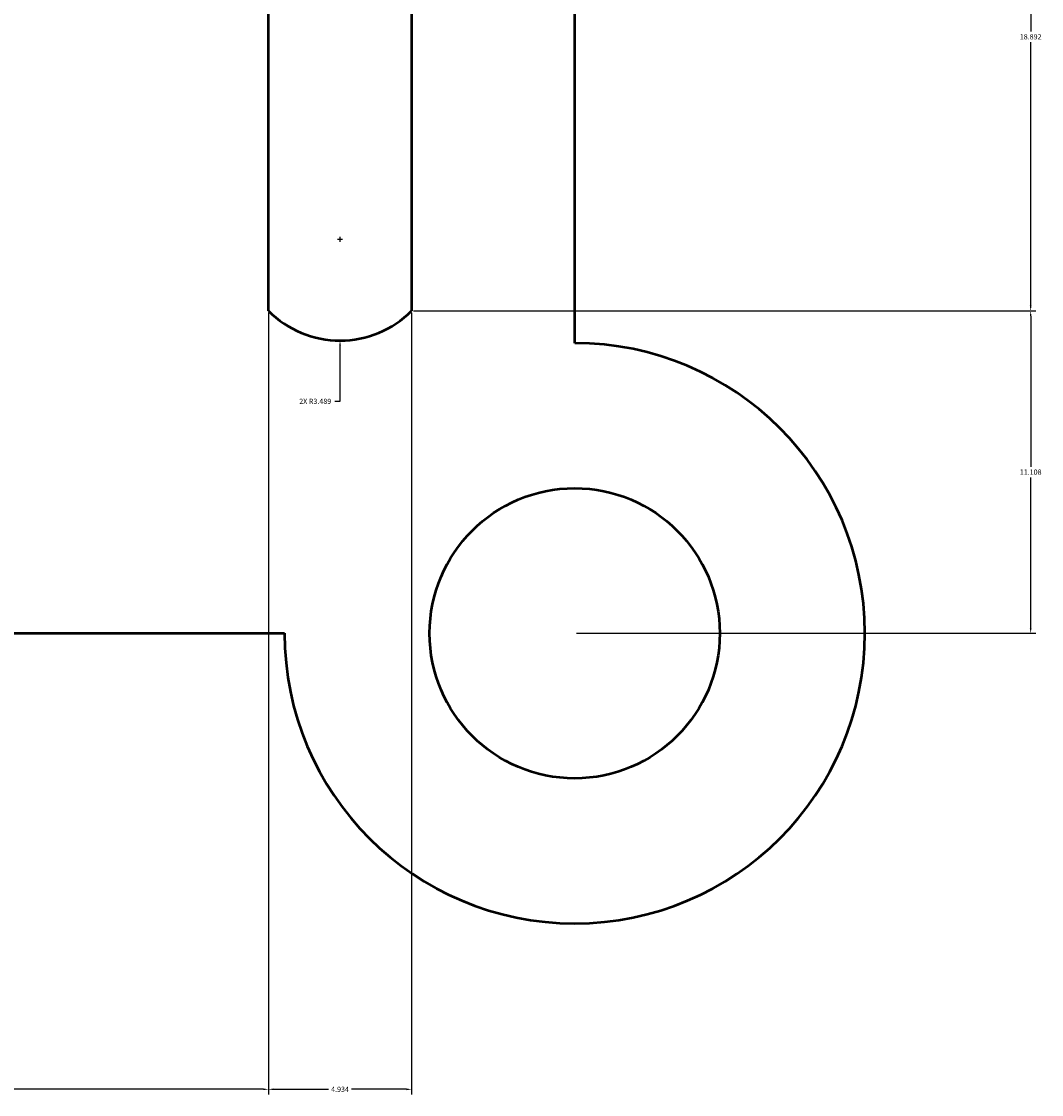
# Model space of a CAD drawing. Units: inches. Extents: x -14 to 108, y -9 to 83.
# Tile 8 of 13: x 73 to 108, y -9 to 28. Entities that reach past the tile are written whole.
import ezdxf

# ---------------------------------------------------------------- set-up
doc = ezdxf.new("R2010")
doc.units = ezdxf.units.IN
doc.header["$MEASUREMENT"] = 0
doc.layers.add('M-DIMS', color=2, linetype='Continuous', lineweight=18)
doc.layers.add('M-OUTL', color=7, linetype='Continuous', lineweight=50)
doc.styles.get("Standard").update_dxf_attribs({"font": 'arial.ttf'})
doc.dimstyles.get("Standard").update_dxf_attribs({"dimtxt": 0.18, "dimasz": 0.18, "dimexe": 0.18, "dimexo": 0.0625, "dimgap": 0.09, "dimtad": 0, "dimtih": 1, "dimtoh": 1, "dimzin": 0, "dimdsep": 46, "dimtxsty": 'Standard', "dimcen": 0.09, "dimadec": 0, "dimazin": 0, "dimtfac": 1, "dimtofl": 0, "dimtmove": 0, "dimatfit": 3, "dimfxl": 1, "dimtolj": 1, "dimtzin": 0, "dimarcsym": 0})

# ---------------------------------------------------------------- blocks, each defined once
blk = doc.blocks.new('SLOT-VERTICAL')
for points in [[(0, 1.021), (0, 40.458)], [(4.933, 40.458), (4.933, 1.021)]]:
    blk.add_lwpolyline(points)
blk.add_arc((2.466, 3.488), 3.489, 225, 315)
blk = doc.blocks.new('HOLE-D10')
blk.add_circle((5, 5), 5)
blk = doc.blocks.new('*D8')
at = {"layer": 'Defpoints', "color": 0, "transparency": 16777216}
for p in [(47.098, 37.119), (81.545, 18.227), (81.545, -8.596)]:
    blk.add_point(p, dxfattribs=at)
at = {"layer": 'M-DIMS', "color": 0, "lineweight": -2, "transparency": 16777216}
for p, q in [((47.098, 37.057), (47.098, -8.776)), ((81.545, 18.165), (81.545, -8.776)), ((47.278, -8.596), (63.927, -8.596)), ((81.365, -8.596), (64.716, -8.596))]:
    blk.add_line(p, q, dxfattribs=at)
at = {"layer": 'M-DIMS', "color": 0, "transparency": 16777216}
for points in [[(47.278, -8.566), (47.278, -8.626), (47.098, -8.596)], [(81.365, -8.566), (81.365, -8.626), (81.545, -8.596)]]:
    blk.add_solid(points, dxfattribs=at)
at = {"layer": 'M-DIMS', "color": 0, "transparency": 16777216, "insert": (64.321, -8.596), "char_height": 0.18, "attachment_point": 5}
blk.add_mtext('\\A1;34.45', dxfattribs=at)
blk = doc.blocks.new('*D9')
at = {"layer": 'Defpoints', "color": 0, "transparency": 16777216}
for p in [(81.545, 18.227), (86.478, 18.227), (86.478, -8.596)]:
    blk.add_point(p, dxfattribs=at)
at = {"layer": 'M-DIMS', "color": 0, "lineweight": -2, "transparency": 16777216}
for p, q in [((81.545, 18.165), (81.545, -8.776)), ((86.478, 18.165), (86.478, -8.776)), ((81.725, -8.596), (83.615, -8.596)), ((86.298, -8.596), (84.408, -8.596))]:
    blk.add_line(p, q, dxfattribs=at)
at = {"layer": 'M-DIMS', "color": 0, "transparency": 16777216}
for points in [[(81.725, -8.566), (81.725, -8.626), (81.545, -8.596)], [(86.298, -8.566), (86.298, -8.626), (86.478, -8.596)]]:
    blk.add_solid(points, dxfattribs=at)
at = {"layer": 'M-DIMS', "color": 0, "transparency": 16777216, "insert": (84.011, -8.596), "char_height": 0.18, "attachment_point": 5}
blk.add_mtext('\\A1;4.934', dxfattribs=at)
blk = doc.blocks.new('*D10')
at = {"layer": 'Defpoints', "color": 0, "transparency": 16777216}
for p in [(86.478, 18.227), (107.813, 18.227), (92.098, 7.119)]:
    blk.add_point(p, dxfattribs=at)
at = {"layer": 'M-DIMS', "color": 0, "lineweight": -2, "transparency": 16777216}
for p, q in [((86.541, 18.227), (107.993, 18.227)), ((107.813, 18.047), (107.813, 12.855)), ((107.813, 7.299), (107.813, 12.491)), ((92.16, 7.119), (107.993, 7.119))]:
    blk.add_line(p, q, dxfattribs=at)
at = {"layer": 'M-DIMS', "color": 0, "transparency": 16777216}
for points in [[(107.783, 18.047), (107.843, 18.047), (107.813, 18.227)], [(107.783, 7.299), (107.843, 7.299), (107.813, 7.119)]]:
    blk.add_solid(points, dxfattribs=at)
at = {"layer": 'M-DIMS', "color": 0, "transparency": 16777216, "insert": (107.813, 12.673), "char_height": 0.18, "attachment_point": 5}
blk.add_mtext('\\A1;11.108', dxfattribs=at)
blk = doc.blocks.new('*D11')
at = {"layer": 'Defpoints', "color": 0, "transparency": 16777216}
for p in [(47.098, 37.119), (107.813, 37.119), (86.478, 18.227)]:
    blk.add_point(p, dxfattribs=at)
at = {"layer": 'M-DIMS', "color": 0, "lineweight": -2, "transparency": 16777216}
for p, q in [((47.16, 37.119), (107.993, 37.119)), ((107.813, 36.939), (107.813, 27.855)), ((107.813, 18.407), (107.813, 27.491)), ((86.541, 18.227), (107.993, 18.227))]:
    blk.add_line(p, q, dxfattribs=at)
at = {"layer": 'M-DIMS', "color": 0, "transparency": 16777216}
for points in [[(107.783, 36.939), (107.843, 36.939), (107.813, 37.119)], [(107.783, 18.407), (107.843, 18.407), (107.813, 18.227)]]:
    blk.add_solid(points, dxfattribs=at)
at = {"layer": 'M-DIMS', "color": 0, "transparency": 16777216, "insert": (107.813, 27.673), "char_height": 0.18, "attachment_point": 5}
blk.add_mtext('\\A1;18.892', dxfattribs=at)
blk = doc.blocks.new('*D26')
at = {"layer": 'Defpoints', "color": 0, "transparency": 16777216}
for p in [(84.011, 20.694), (84.011, 17.206)]:
    blk.add_point(p, dxfattribs=at)
at = {"layer": 'M-DIMS', "color": 0, "lineweight": -2, "transparency": 16777216}
for p, q in [((84.011, 20.604), (84.011, 20.784)), ((83.921, 20.694), (84.101, 20.694)), ((84.011, 15.112), (84.011, 17.026)), ((83.831, 15.112), (84.011, 15.112))]:
    blk.add_line(p, q, dxfattribs=at)
at = {"layer": 'M-DIMS', "color": 0, "transparency": 16777216}
blk.add_solid([(83.981, 17.026), (84.041, 17.026), (84.011, 17.206)], dxfattribs=at)
at = {"layer": 'M-DIMS', "color": 0, "transparency": 16777216, "insert": (83.156, 15.112), "char_height": 0.18, "attachment_point": 5}
blk.add_mtext('\\A1;2X R3.489', dxfattribs=at)

msp = doc.modelspace()

# ---------------------------------------------------------------- linework, layer by layer
at = {"layer": 'M-OUTL'}
for points in [[(92.0979, 17.1193), (92.0979, 57.1193)], [(12.0979, 7.1193), (82.0979, 7.1193)]]:
    msp.add_lwpolyline(points, dxfattribs=at)
msp.add_arc((92.0979, 7.1193), 10, 180, 90, dxfattribs=at)

# ---------------------------------------------------------------- block references
for name, p in [('SLOT-VERTICAL', (81.545, 17.206)), ('HOLE-D10', (87.098, 2.119))]:
    msp.add_blockref(name, p, dxfattribs=at)

# ---------------------------------------------------------------- dimensions: what is measured, and where the dimension line sits
at = {"layer": 'M-DIMS'}
for base, p1, p2, override, picture, middle in [((81.5446, -8.5957), (47.0979, 37.1193), (81.5446, 18.2274), {"dimdec": 2, "dimlfac": 1, "dimrnd": 0, "dimzin": 0, "dimdsep": 46, "dimlunit": 2}, '*D8', (64.3213, -8.5957)), ((86.4784, -8.5957), (81.5446, 18.2274), (86.4784, 18.2274), {"dimdec": 3, "dimlfac": 1, "dimrnd": 0, "dimzin": 0, "dimdsep": 46, "dimlunit": 2}, '*D9', (84.0115, -8.5957))]:
    dim = msp.add_linear_dim(base=base, p1=p1, p2=p2, dimstyle='Standard', override=override, dxfattribs=at)
    dim.commit()
    dim.dimension.update_dxf_attribs({"geometry": picture, "text_midpoint": middle})
for base, p1, p2, picture, middle in [((107.8129, 37.1193), (86.4784, 18.2274), (47.0979, 37.1193), '*D11', (107.8129, 27.6733)), ((107.8129, 18.2274), (92.0979, 7.1193), (86.4784, 18.2274), '*D10', (107.8129, 12.6733))]:
    dim = msp.add_linear_dim(base=base, p1=p1, p2=p2, angle=90, dimstyle='Standard', override={"dimdec": 3, "dimlfac": 1, "dimrnd": 0, "dimzin": 0, "dimdsep": 46, "dimlunit": 2}, dxfattribs=at)
    dim.commit()
    dim.dimension.update_dxf_attribs({"geometry": picture, "text_midpoint": middle})
dim = msp.add_radius_dim(center=(84.0115, 20.6942), mpoint=(84.011, 17.2056), text='2X <>', dimstyle='Standard', override={"dimdec": 3, "dimlfac": 1, "dimrnd": 0, "dimzin": 0, "dimdsep": 46, "dimlunit": 2}, dxfattribs=at)
dim.commit()
dim.dimension.update_dxf_attribs({"geometry": '*D26', "text_midpoint": (83.1558, 15.1124), "dimtype": 164})

doc.saveas('drawing.dxf')
